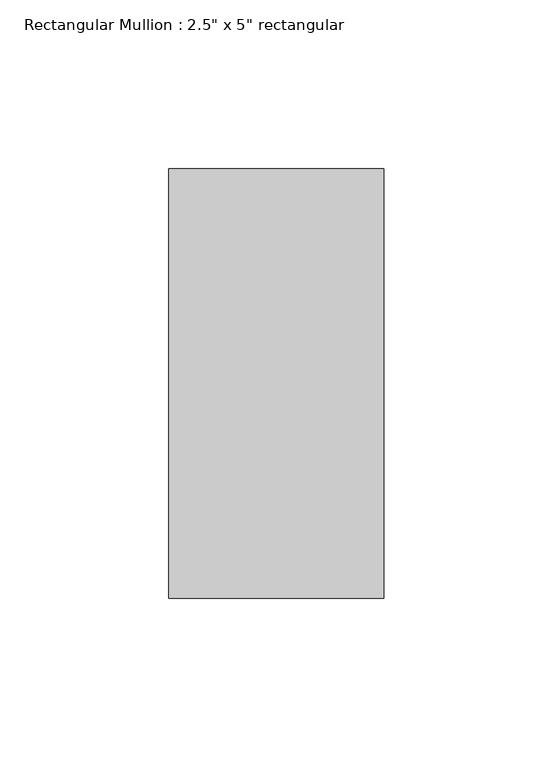
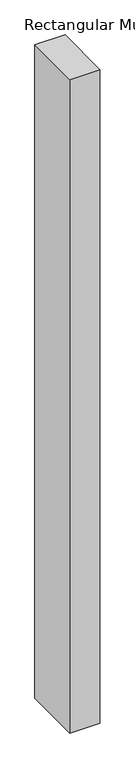
"""IFC4 building model written with IfcOpenShell, lengths in millimetres: member geometry."""

from ifc_helpers import new_model, si_unit, frame, origin, place, context, project, spatial, polyline, outline, extrude, source, transform, mapped, element, save


def member_9dfa5507(model_context):
    return source(origin(), model_context, "Body", "SweptSolid", [
        extrude(outline(polyline([(0.0, 63.5), (0.0, -63.5), (-63.5, -63.5), (-63.5, 63.5), (0.0, 63.5)])), frame((0.0, 0.0, -1454.3964565), z_axis=(0.0, 0.0, 1.0), x_axis=(1.0, 0.0, 0.0)), (0.0, 0.0, 1.0), 1454.3964565),
    ])


if __name__ == "__main__":
    model = new_model("IFC4")
    model_context = context("Model", 3, world=origin())
    ifc_project = project(units=[si_unit("LENGTHUNIT", "METRE", prefix="MILLI")], contexts=[model_context])
    site = spatial("IfcSite", under=ifc_project)
    building = spatial("IfcBuilding", under=site)
    placement = place(None, origin())
    member_shape = member_9dfa5507(model_context)
    element("IfcMember", 1, ObjectType="Rectangular Mullion : 2.5\" x 5\" rectangular", at=placement, inside=building, context=model_context, shape_type="MappedRepresentation", body=[
        mapped(member_shape, transform((0.0, 0.0, 0.0), x_axis=(1.0, 0.0, 0.0), y_axis=(0.0, 1.0, 0.0), z_axis=(0.0, 0.0, 1.0))),
    ])
    save(model, "model.ifc")

# Revit data of these elements
# Type "Rectangular Mullion : 2.5\" x 5\" rectangular"
#   built-in parameter 1007304 = 0.416667 (stored number, unit not read)
#   built-in parameter 1007301 = 0.104167 (stored number, unit not read)
#   built-in parameter 1007300 = 0.104167 (stored number, unit not read)
# Element 1 (IfcMember, "Rectangular Mullion : 2.5\" x 5\" rectangular")
#   Materials on its faces: "Aluminum"
# Materials
#   "Aluminum": class "Metal", colour RGB 247 247 247, transparency 0, Description = "Aluminum 6061", Cost = 0
